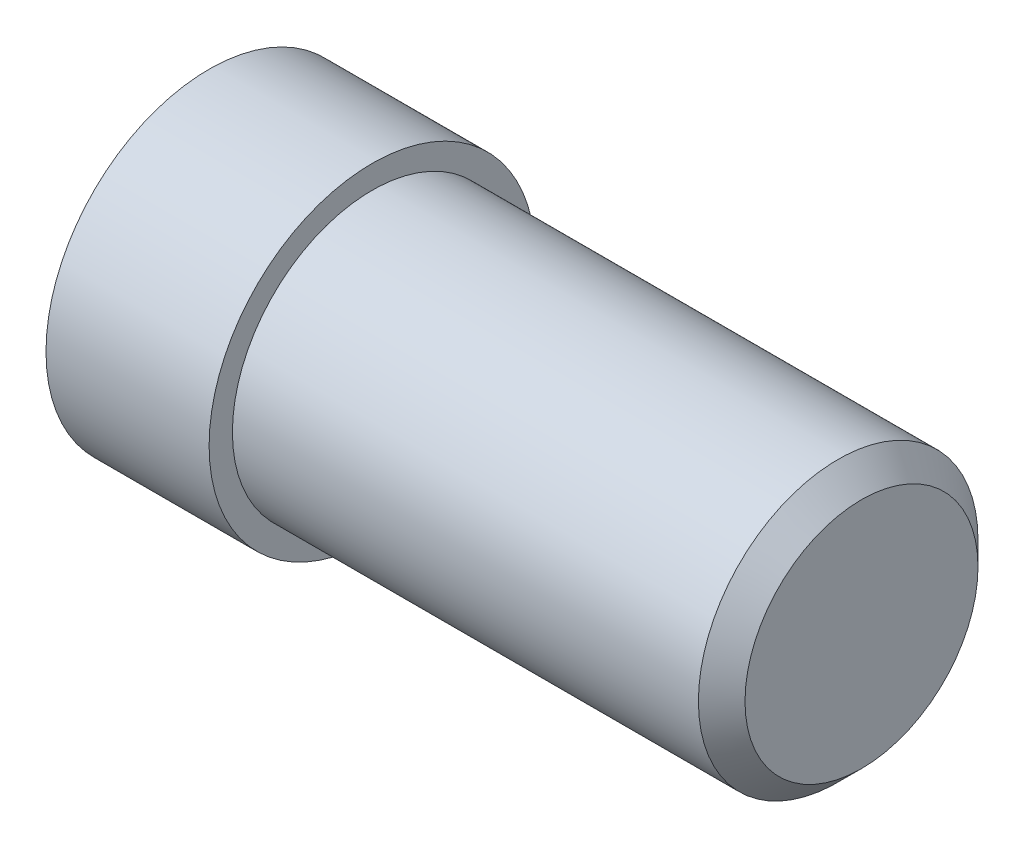
from build123d import *

# Parameters (mm, degrees)
SHANK_TIP_CHAMFER_1X45_SIZE = 1


with BuildPart() as part:
    # Bolt Profile Sketch → Bolt Body Revolve (revolve)
    with BuildSketch(Plane.XY, mode=Mode.PRIVATE) as bolt_body_revolve_sk:
        Polygon((0, 0), (21, 0), (21, 6), (0, 6), (0, 7), (-7, 7), (-7, 0), align=None)
    revolve(bolt_body_revolve_sk.sketch.rotate(Axis((0, 0, 0), (1, 0, 0)), 90), axis=Axis((0, 0, 0), (1, 0, 0)))

    # Shank Tip Chamfer 1x45°
    shank_tip_chamfer_1x45_edges = [part.edges().sort_by_distance(p)[0] for p in [
        (21, 0, -6),
    ]]
    chamfer(shank_tip_chamfer_1x45_edges, length=SHANK_TIP_CHAMFER_1X45_SIZE)


solid = part.part
